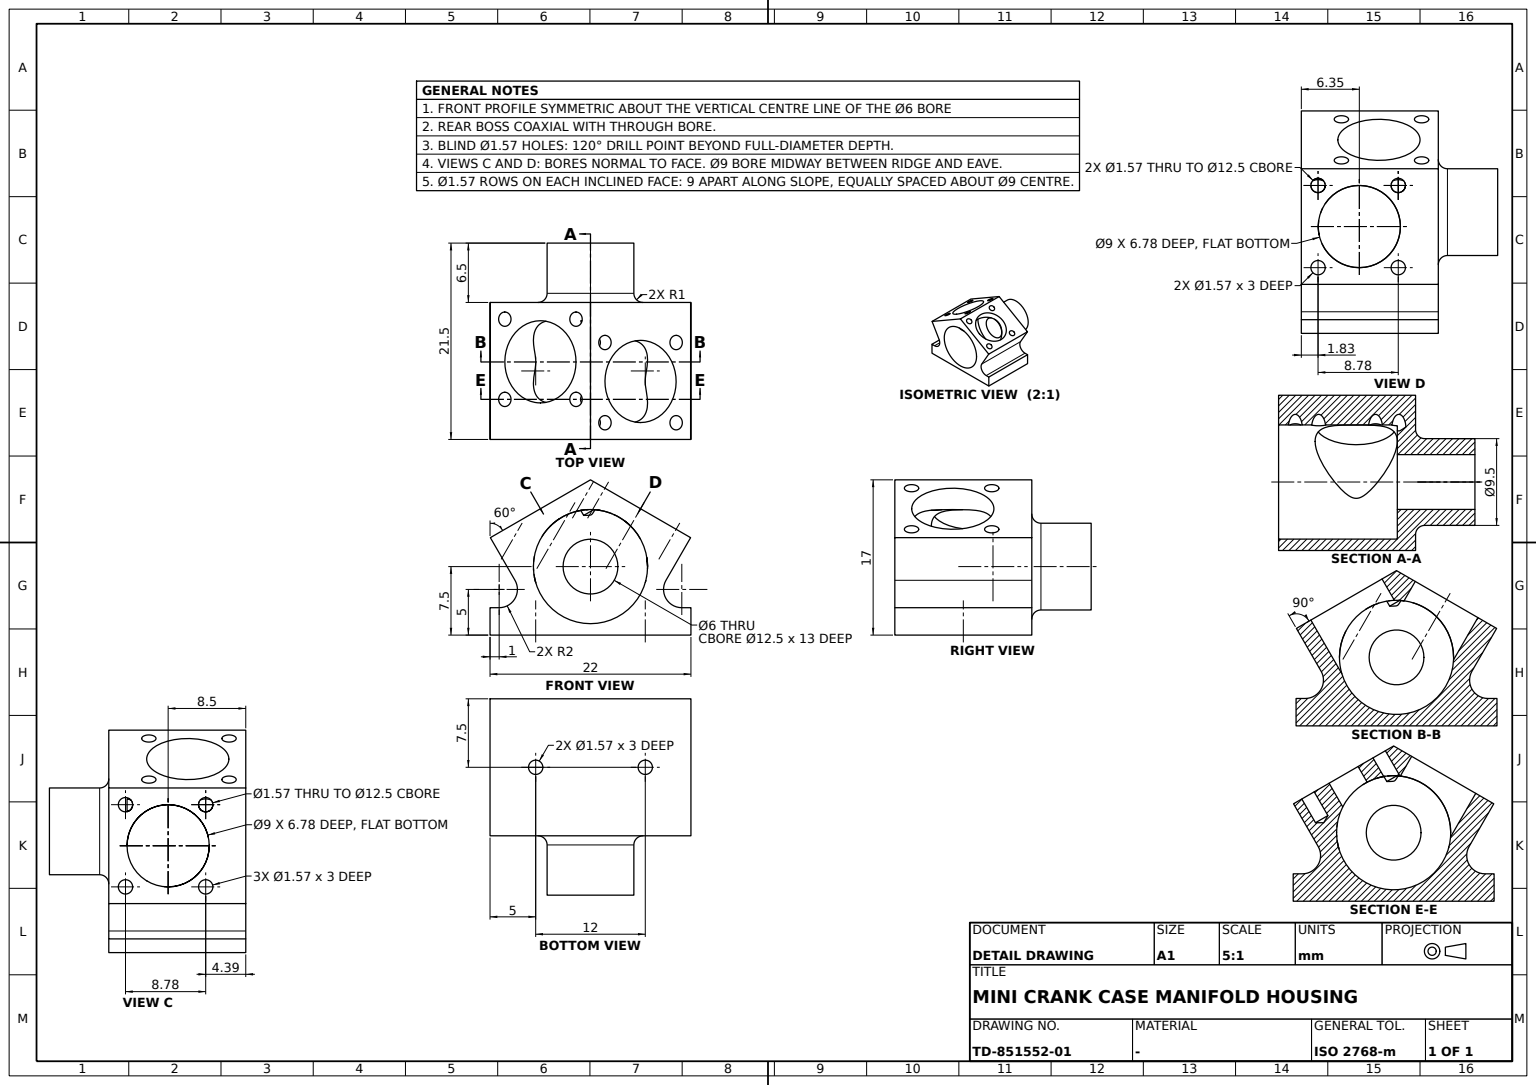
CATIA V5 part; units mm, degrees
sketch "Sketch1" plane through (0, 0, 0) normal (1, 0, 0) x (0, 1, 0)
  line L0 (-11, 0) -> (11, 0)
  line L1 (-11, 0) -> (-11, 3)
  line L2 (11, 0) -> (11, 3)
  line L3 (-11, 3) -> (-10, 3)
  line L4 (11, 3) -> (10, 3)
  arc A0 (8.2679, 6) -> (10, 3) centre (10, 5) ccw
  point P0 (10, 5)
  point P1 (11, 6.7321)
  arc A1 (-10, 3) -> (-8.2679, 6) centre (-10, 5) ccw
  point P2 (-10, 5)
  line L5 (0, 17) -> (-10.9641, 10.6699)
  point P3 (0, 17)
  point P4 (-10.9641, 10.6699)
  line L6 (-10.9641, 10.6699) -> (-8.2679, 6)
  point P5 (-10.9641, 10.6699)
  line L7 (0, 17) -> (10.9641, 10.6699)
  point P6 (10.9641, 10.6699)
  line L8 (10.9641, 10.6699) -> (8.2679, 6)
  point P7 (10.9641, 10.6699)
  dimension "length L0" = 22
  dimension "length L1" = 3
  dimension "length L2" = 3
  dimension "distance P0 L0" = 5
  dimension "distance P0 L2" = 1
  dimension "radius A0" = 2
  dimension "radius A1" = 2
  dimension "distance P2 L0" = 5
  dimension "distance P2 L1" = 1
  dimension "angle L5 L0" = 30
  dimension "distance P3 L0" = 17
  dimension "angle L7 L0" = 30
  constraint midpoint L0 origin
  constraint horizontal L0 x-axis
  constraint horizontal L3 x-axis
  constraint horizontal L4 x-axis
  constraint vertical L1 y-axis
  constraint vertical L2 y-axis
  constraint coincidence A0 P1
  constraint coincidence P1 L2
  constraint coincidence P3 y-axis
  constraint coincidence P5 L5
  constraint coincidence P4 L6
  constraint coincidence P6 L8
  constraint coincidence P7 L7
  constraint coincidence P4 P5
  constraint coincidence P6 P7
  constraint perpendicularity L6 L5
  constraint perpendicularity L8 L7
  constraint tangency L6 A1
  constraint tangency L8 A0
extrude "Pad1" add sketch "Sketch1" along normal mid plane 15
sketch "Sketch2" plane through (-7.5, 0, 0) normal (-1, 0, 0) x (0, -1, 0)
  circle A0 centre (0, 7.5) radius 4.75
  point P0 (0, 7.5)
  line L0 (11, 0) -> (-11, 0) construction
  dimension "distance P0 L0" = 7.5
  dimension "radius A0" = 4.75
  constraint coincidence P0 y-axis
extrude "Pad2" add sketch "Sketch2" along normal blind 6.5
sketch "Sketch3" plane through (7.5, 0, 0) normal (1, 0, 0) x (0, 1, 0)
  circle A0 centre (0, 7.5) radius 6.25
  point P0 (0, 7.5)
  line L0 (-11, 0) -> (11, 0) construction
  dimension "radius A0" = 6.25
  dimension "distance P0 L0" = 7.5
  constraint coincidence P0 y-axis
extrude "Pocket1" cut sketch "Sketch3" against normal blind 13
sketch "Sketch4" plane through (-14, 0, 0) normal (-1, 0, 0) x (0, -1, 0)
  circle A0 centre (0, 7.5) radius 3
  point P0 (0, 7.5)
  circle A1 centre (0, 7.5) radius 4.75 construction
  dimension "radius A0" = 3
  constraint coincidence P0 y-axis
  constraint concentricity A0 A1
extrude "Pocket2" cut sketch "Sketch4" against normal through all
fillet "Fillet1" radius 1 1 edges at (-7.5, 4.75, 7.5)
sketch "Sketch5" plane through (-1.8293, 8.599, 0) normal (0, 0, -1) x (1, 0, 0)
  point P0 (1.8293, 2.599)
  line L0 (-5.6707, 19.599) -> (-5.6707, -2.401) construction
  dimension "D1" = 6
  dimension "distance P0 L0" = 7.5
hole "Hole1" at (0, 6, 0) direction (0, 0, 1) diameter 1.567 depth 3 tip angle 120 thread major 2 thread length 3 thread pitch 0.4
sketch "Sketch6" plane through (-1.3726, -5.6156, 0) normal (0, 0, -1) x (1, 0, 0)
  point P0 (1.3726, 0.3844)
  line L0 (8.8726, 5.3844) -> (8.8726, -16.6156) construction
  line L1 (-6.1274, 5.3844) -> (8.8726, 5.3844) construction
  dimension "distance P0 L0" = 7.5
  dimension "distance P0 L1" = 5
hole "Hole2" at (0, -6, 0) direction (0, 0, 1) diameter 1.567 depth 3 tip angle 120 thread major 2 thread length 3 thread pitch 0.4
sketch "Sketch7" plane through (0, 7.3612, 12.75) normal (0, 0.5, 0.866) x (-1, 0, 0)
  circle A0 centre (-1.15, 2.17) radius 4.5
  point P0 (-1.15, 2.17)
  line L0 (7.5, 8.5) -> (-7.5, 8.5) construction
  line L1 (-7.5, -4.1603) -> (-7.5, 8.5) construction
  dimension "distance P0 L0" = 6.33
  dimension "distance P0 L1" = 6.35
  dimension "radius A0" = 4.5
extrude "Pocket3" cut sketch "Sketch7" against normal up to next
sketch "Sketch8" plane through (-5.549, 8.9359, 11.8408) normal (0, 0.5, 0.866) x (1, 0, 0)
  point P0 (11.219, 0.5119)
  line L0 (13.049, 2.3419) -> (13.049, -10.3183) construction
  line L1 (-1.951, 2.3419) -> (13.049, 2.3419) construction
  dimension "distance P0 L0" = 1.83
  dimension "distance P0 L1" = 1.83
hole "Hole3" at (5.67, 9.3793, 11.5849) direction (0, -0.5, -0.866) diameter 1.567 depth 3 tip angle 120 thread major 2 thread length 3 thread pitch 0.4
sketch "Sketch9" plane through (-4.7873, 9.3035, 11.6286) normal (0, 0.5, 0.866) x (1, 0, 0)
  point P0 (1.6738, 0.0875)
  line L0 (-2.7127, 1.9175) -> (12.2873, 1.9175) construction
  circle A0 centre (10.4573, 0.0875) radius 0.7835 construction
  dimension "distance P0 L0" = 1.83
  dimension "distance A0 P0" = 8
hole "Hole4" at (-3.1135, 9.3793, 11.5849) direction (0, -0.5, -0.866) diameter 1.567 depth 3 tip angle 120 thread major 2 thread length 3 thread pitch 0.4
sketch "Sketch10" plane through (5.3928, 1.8134, 15.9531) normal (0, 0.5, 0.866) x (1, 0, 0)
  point P0 (0.2772, -0.2639)
  line L0 (2.1072, 10.5664) -> (2.1072, -2.0939) construction
  line L1 (-12.8928, -2.0939) -> (2.1072, -2.0939) construction
  dimension "distance P0 L0" = 1.83
  dimension "distance P0 L1" = 1.83
hole "Hole5" at (5.67, 1.5848, 16.085) direction (0, -0.5, -0.866) diameter 1.567 depth 3 tip angle 120 thread major 2 thread length 3 thread pitch 0.4
sketch "Sketch11" plane through (-4.8592, 2.7451, 15.4151) normal (0, 0.5, 0.866) x (1, 0, 0)
  point P0 (1.7457, -1.3398)
  line L0 (-2.6408, -3.1698) -> (12.3592, -3.1698) construction
  circle A0 centre (10.5292, -1.3398) radius 0.7835 construction
  dimension "distance P0 L0" = 1.83
  dimension "distance A0 P0" = 8
hole "Hole6" at (-3.1135, 1.5848, 16.085) direction (0, -0.5, -0.866) diameter 1.567 depth 3 tip angle 120 thread major 2 thread length 3 thread pitch 0.4
sketch "Sketch12" plane through (0, -7.3612, 12.75) normal (0, -0.5, 0.866) x (1, 0, 0)
  circle A0 centre (-1, 2.1697) radius 4.5
  point P0 (-1, 2.1697)
  line L0 (-7.5, -4.1603) -> (7.5, -4.1603) construction
  line L1 (-7.5, 8.5) -> (-7.5, -4.1603) construction
  dimension "distance P0 L0" = 6.33
  dimension "distance P0 L1" = 6.5
  dimension "radius A0" = 4.5
extrude "Pocket4" cut sketch "Sketch12" against normal up to next
sketch "Sketch13" plane through (-5.3934, -2.2359, 15.7091) normal (0, -0.5, 0.866) x (1, 0, 0)
  point P0 (-0.2766, 0.7518)
  line L0 (-2.1066, 2.5818) -> (-2.1066, -10.0785) construction
  line L1 (-2.1066, 2.5818) -> (12.8934, 2.5818) construction
  dimension "distance P0 L0" = 1.83
  dimension "distance P0 L1" = 1.83
hole "Hole7" at (-5.67, -1.5848, 16.085) direction (0, 0.5, -0.866) diameter 1.567 depth 3 tip angle 120 thread major 2 thread length 3 thread pitch 0.4
sketch "Sketch14" plane through (3.2318, -1.439, 16.1692) normal (0, -0.5, 0.866) x (1, 0, 0)
  point P0 (-0.1183, -0.1684)
  line L0 (-10.7318, 1.6616) -> (4.2682, 1.6616) construction
  circle A0 centre (-8.9018, -0.1684) radius 0.7835 construction
  dimension "distance P0 L0" = 1.83
  dimension "distance A0 P0" = 8
hole "Hole8" at (3.1135, -1.5848, 16.085) direction (0, 0.5, -0.866) diameter 1.567 depth 3 tip angle 120 thread major 2 thread length 3 thread pitch 0.4
sketch "Sketch15" plane through (-5.0944, -9.4351, 11.5526) normal (0, -0.5, 0.866) x (1, 0, 0)
  point P0 (-0.5756, 0.0645)
  line L0 (-2.4056, -1.7655) -> (12.5944, -1.7655) construction
  line L1 (-2.4056, 10.8948) -> (-2.4056, -1.7655) construction
  dimension "distance P0 L0" = 1.83
  dimension "distance P0 L1" = 1.83
hole "Hole9" at (-5.67, -9.3793, 11.5849) direction (0, 0.5, -0.866) diameter 1.567 depth 3 tip angle 120 thread major 2 thread length 3 thread pitch 0.4
sketch "Sketch16" plane through (3.6552, -10.0638, 11.1897) normal (0, -0.5, 0.866) x (1, 0, 0)
  point P0 (-0.5417, 0.7904)
  line L0 (-11.1552, -1.0396) -> (3.8448, -1.0396) construction
  circle A0 centre (-9.3252, 0.7904) radius 0.7835 construction
  dimension "distance P0 L0" = 1.83
  dimension "distance A0 P0" = 8
hole "Hole10" at (3.1135, -9.3793, 11.5849) direction (0, 0.5, -0.866) diameter 1.567 depth 3 tip angle 120 thread major 2 thread length 3 thread pitch 0.4
